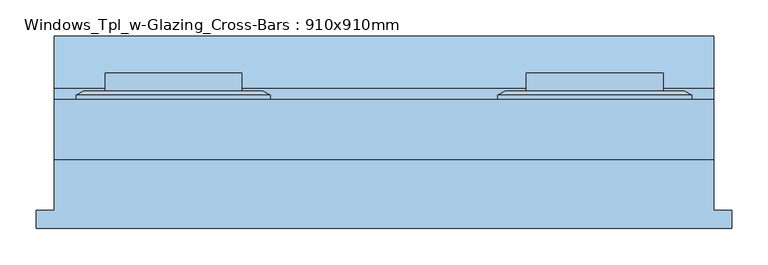
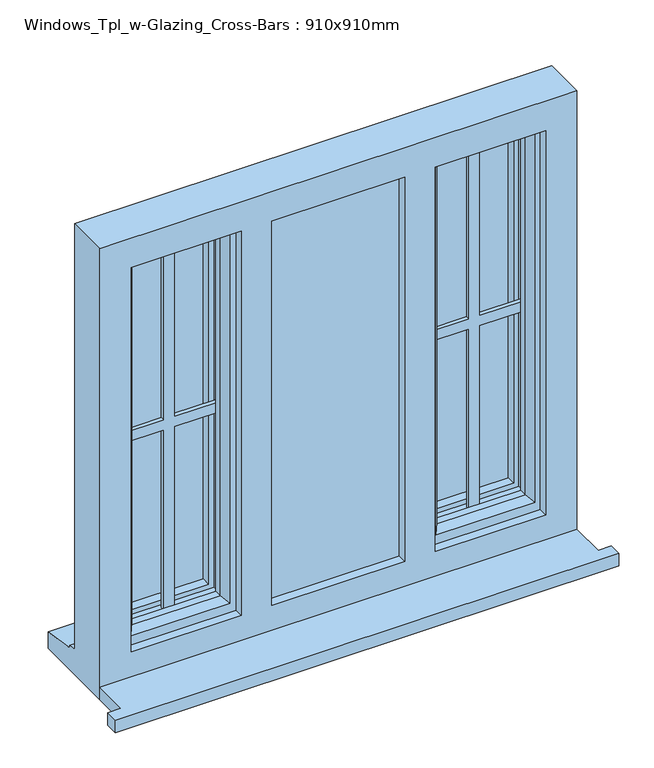
"""IFC4 building model written with IfcOpenShell, lengths in millimetres: window geometry, Windows_Tpl_w-Glazing_Cross-Bars : 910x910mm."""

from ifc_helpers import new_model, si_unit, frame, origin, place, context, project, spatial, polyline, outline, extrude, faceted_brep, source, transform, mapped, element, save


def windows_tpl_w_glazing_cross_bars_910x910mm_4aa0f884(model_context):
    return source(origin(), model_context, "Body", "SolidModel", [
        extrude(outline(polyline([(-906.6666667, -118.1434322), (-906.6666667, -93.1434322), (-881.6666667, -93.1434322), (-881.6666667, -22.9434322), (28.3333333, -22.9434322), (28.3333333, -93.1434322), (53.3333333, -93.1434322), (53.3333333, -118.1434322), (-906.6666667, -118.1434322)])), frame((0.0, 0.0, 1200.0), z_axis=(0.0, 0.0, 1.0), x_axis=(1.0, 0.0, 0.0)), (0.0, 0.0, 1.0), 25.0),
        faceted_brep([(-270.0, 60.0565678, 2080.0), (-270.0, 65.8300705, 2080.0), (-270.0, 65.8300705, 1253.0), (-270.0, 60.0565678, 1253.0), (-260.0, -4.9434322, 2070.0), (-260.0, 60.0565678, 2070.0), (-260.0, 60.0565678, 1263.0), (-260.0, -4.9434322, 1263.0), (-220.0, 9.5494677, 2030.0), (-230.1480377, -4.9434322, 2040.1480377), (-230.1480377, -4.9434322, 1292.8519623), (-220.0, 9.5494677, 1303.0), (-220.0, 24.0565678, 2030.0), (-220.0, 24.0565678, 1303.0), (-230.0, 48.0565678, 2040.0), (-230.0, 24.0565678, 2040.0), (-230.0, 24.0565678, 1293.0), (-230.0, 48.0565678, 1293.0), (-220.0, 65.8300705, 2030.0), (-220.0, 48.0565678, 2030.0), (-220.0, 48.0565678, 1303.0), (-220.0, 65.8300705, 1303.0), (-237.4457548, 71.6035732, 2047.4457548), (-237.4457548, 71.6035732, 1285.5542452), (-259.2153903, 71.6035732, 2069.2153903), (-259.2153903, 71.6035732, 1263.7846097), (-1.6666667, 65.8300705, 1253.0), (-1.6666667, 60.0565678, 1253.0), (-11.6666667, 60.0565678, 1263.0), (-11.6666667, -4.9434322, 1263.0), (-41.5186289, -4.9434322, 1292.8519623), (-51.6666667, 9.5494677, 1303.0), (-51.6666667, 24.0565678, 1303.0), (-41.6666667, 24.0565678, 1293.0), (-41.6666667, 48.0565678, 1293.0), (-51.6666667, 48.0565678, 1303.0), (-51.6666667, 65.8300705, 1303.0), (-34.2209119, 71.6035732, 1285.5542452), (-12.4512764, 71.6035732, 1263.7846097), (-1.6666667, 65.8300705, 2080.0), (-1.6666667, 60.0565678, 2080.0), (-11.6666667, 60.0565678, 2070.0), (-11.6666667, -4.9434322, 2070.0), (-41.5186289, -4.9434322, 2040.1480377), (-51.6666667, 9.5494677, 2030.0), (-51.6666667, 24.0565678, 2030.0), (-41.6666667, 24.0565678, 2040.0), (-41.6666667, 48.0565678, 2040.0), (-51.6666667, 48.0565678, 2030.0), (-51.6666667, 65.8300705, 2030.0), (-34.2209119, 71.6035732, 2047.4457548), (-12.4512764, 71.6035732, 2069.2153903)], [[[0, 1, 2, 3]], [[4, 5, 6, 7]], [[8, 9, 10, 11]], [[12, 8, 11, 13]], [[14, 15, 16, 17]], [[18, 19, 20, 21]], [[22, 18, 21, 23]], [[1, 24, 25, 2]], [[3, 2, 26, 27]], [[7, 6, 28, 29]], [[11, 10, 30, 31]], [[13, 11, 31, 32]], [[17, 16, 33, 34]], [[21, 20, 35, 36]], [[23, 21, 36, 37]], [[2, 25, 38, 26]], [[27, 26, 39, 40]], [[29, 28, 41, 42]], [[31, 30, 43, 44]], [[32, 31, 44, 45]], [[34, 33, 46, 47]], [[36, 35, 48, 49]], [[37, 36, 49, 50]], [[26, 38, 51, 39]], [[40, 39, 1, 0]], [[3, 27, 40, 0], [5, 41, 28, 6]], [[42, 41, 5, 4]], [[7, 29, 42, 4], [9, 43, 30, 10]], [[44, 43, 9, 8]], [[45, 44, 8, 12]], [[15, 46, 33, 16], [13, 32, 45, 12]], [[47, 46, 15, 14]], [[17, 34, 47, 14], [19, 48, 35, 20]], [[49, 48, 19, 18]], [[50, 49, 18, 22]], [[24, 51, 38, 25], [23, 37, 50, 22]], [[39, 51, 24, 1]]]),
        faceted_brep([(-583.3333333, 60.0565678, 2080.0), (-583.3333333, 65.8300705, 2080.0), (-851.6666667, 65.8300705, 2080.0), (-851.6666667, 60.0565678, 2080.0), (-593.3333333, -4.9434322, 2070.0), (-593.3333333, 60.0565678, 2070.0), (-841.6666667, 60.0565678, 2070.0), (-841.6666667, -4.9434322, 2070.0), (-633.3333333, 9.5494677, 2030.0), (-623.1852956, -4.9434322, 2040.1480377), (-811.8147044, -4.9434322, 2040.1480377), (-801.6666667, 9.5494677, 2030.0), (-633.3333333, 24.0565678, 2030.0), (-801.6666667, 24.0565678, 2030.0), (-623.3333333, 48.0565678, 2040.0), (-623.3333333, 24.0565678, 2040.0), (-811.6666667, 24.0565678, 2040.0), (-811.6666667, 48.0565678, 2040.0), (-633.3333333, 65.8300705, 2030.0), (-633.3333333, 48.0565678, 2030.0), (-801.6666667, 48.0565678, 2030.0), (-801.6666667, 65.8300705, 2030.0), (-615.8875785, 71.6035732, 2047.4457548), (-819.1124215, 71.6035732, 2047.4457548), (-594.117943, 71.6035732, 2069.2153903), (-840.882057, 71.6035732, 2069.2153903), (-851.6666667, 65.8300705, 1253.0), (-851.6666667, 60.0565678, 1253.0), (-841.6666667, 60.0565678, 1263.0), (-841.6666667, -4.9434322, 1263.0), (-811.8147044, -4.9434322, 1292.8519623), (-801.6666667, 9.5494677, 1303.0), (-801.6666667, 24.0565678, 1303.0), (-811.6666667, 24.0565678, 1293.0), (-811.6666667, 48.0565678, 1293.0), (-801.6666667, 48.0565678, 1303.0), (-801.6666667, 65.8300705, 1303.0), (-819.1124215, 71.6035732, 1285.5542452), (-840.882057, 71.6035732, 1263.7846097), (-583.3333333, 65.8300705, 1253.0), (-583.3333333, 60.0565678, 1253.0), (-593.3333333, 60.0565678, 1263.0), (-593.3333333, -4.9434322, 1263.0), (-623.1852956, -4.9434322, 1292.8519623), (-633.3333333, 9.5494677, 1303.0), (-633.3333333, 24.0565678, 1303.0), (-623.3333333, 24.0565678, 1293.0), (-623.3333333, 48.0565678, 1293.0), (-633.3333333, 48.0565678, 1303.0), (-633.3333333, 65.8300705, 1303.0), (-615.8875785, 71.6035732, 1285.5542452), (-594.117943, 71.6035732, 1263.7846097)], [[[0, 1, 2, 3]], [[4, 5, 6, 7]], [[8, 9, 10, 11]], [[12, 8, 11, 13]], [[14, 15, 16, 17]], [[18, 19, 20, 21]], [[22, 18, 21, 23]], [[1, 24, 25, 2]], [[3, 2, 26, 27]], [[7, 6, 28, 29]], [[11, 10, 30, 31]], [[13, 11, 31, 32]], [[17, 16, 33, 34]], [[21, 20, 35, 36]], [[23, 21, 36, 37]], [[2, 25, 38, 26]], [[27, 26, 39, 40]], [[0, 3, 27, 40], [41, 28, 6, 5]], [[29, 28, 41, 42]], [[4, 7, 29, 42], [43, 30, 10, 9]], [[31, 30, 43, 44]], [[32, 31, 44, 45]], [[46, 33, 16, 15], [12, 13, 32, 45]], [[34, 33, 46, 47]], [[14, 17, 34, 47], [48, 35, 20, 19]], [[36, 35, 48, 49]], [[37, 36, 49, 50]], [[51, 38, 25, 24], [22, 23, 37, 50]], [[26, 38, 51, 39]], [[40, 39, 1, 0]], [[42, 41, 5, 4]], [[44, 43, 9, 8]], [[45, 44, 8, 12]], [[47, 46, 15, 14]], [[49, 48, 19, 18]], [[50, 49, 18, 22]], [[39, 51, 24, 1]]]),
        extrude(outline(polyline([(1293.0, -145.8333333), (1293.0, -125.8333333), (1656.5, -125.8333333), (1656.5, -41.6666667), (1676.5, -41.6666667), (1676.5, -125.8333333), (2040.1480377, -125.8333333), (2040.1480377, -145.8333333), (1676.5, -145.8333333), (1676.5, -230.1480377), (1656.5, -230.1480377), (1656.5, -145.8333333), (1293.0, -145.8333333)])), frame((0.0, 32.0565678, 0.0), z_axis=(0.0, 1.0, 0.0), x_axis=(0.0, 0.0, 1.0)), (0.0, 0.0, 1.0), 8.0),
        extrude(outline(polyline([(1293.0, -727.5), (1293.0, -707.5), (1656.5, -707.5), (1656.5, -623.3333333), (1676.5, -623.3333333), (1676.5, -707.5), (2040.1480377, -707.5), (2040.1480377, -727.5), (1676.5, -727.5), (1676.5, -811.6666667), (1656.5, -811.6666667), (1656.5, -727.5), (1293.0, -727.5)])), frame((0.0, 32.0565678, 0.0), z_axis=(0.0, 1.0, 0.0), x_axis=(0.0, 0.0, 1.0)), (0.0, 0.0, 1.0), 8.0),
        extrude(outline(polyline([(1263.0, -436.6666667), (1263.0, -416.6666667), (1656.5, -416.6666667), (1656.5, -290.0), (1676.5, -290.0), (1676.5, -416.6666667), (2070.0, -416.6666667), (2070.0, -436.6666667), (1676.5, -436.6666667), (1676.5, -563.3333333), (1656.5, -563.3333333), (1656.5, -436.6666667), (1263.0, -436.6666667)])), frame((0.0, 3.0565678, 0.0), z_axis=(0.0, 1.0, 0.0), x_axis=(0.0, 0.0, 1.0)), (0.0, 0.0, 1.0), 8.0),
        faceted_brep([(28.3333333, -22.9434322, 2110.0), (-881.6666667, -22.9434322, 2110.0), (-881.6666667, -22.9434322, 1200.0), (28.3333333, -22.9434322, 1200.0), (-31.6666667, -22.9434322, 2050.0), (-31.6666667, -22.9434322, 1275.0), (-242.0, -22.9434322, 1275.0), (-242.0, -22.9434322, 2050.0), (-300.0, -22.9434322, 2050.0), (-300.0, -22.9434322, 1275.0), (-553.3333333, -22.9434322, 1275.0), (-553.3333333, -22.9434322, 2050.0), (-611.3333333, -22.9434322, 2050.0), (-611.3333333, -22.9434322, 1275.0), (-821.6666667, -22.9434322, 1275.0), (-821.6666667, -22.9434322, 2050.0), (-881.6666667, 60.0565678, 2110.0), (-881.6666667, 60.0565678, 1251.0), (-881.6666667, 75.0565678, 1249.68767), (-881.6666667, 75.0565678, 1244.7449676), (-881.6666667, 147.5565678, 1233.8088847), (-881.6666667, 147.5565678, 1200.0), (28.3333333, 60.0565678, 2110.0), (28.3333333, 60.0565678, 1251.0), (-841.6666667, 60.0565678, 2070.0), (-841.6666667, 60.0565678, 1263.0), (-593.3333333, 60.0565678, 1263.0), (-593.3333333, 60.0565678, 2070.0), (-553.3333333, 60.0565678, 2070.0), (-553.3333333, 60.0565678, 1263.0), (-300.0, 60.0565678, 1263.0), (-300.0, 60.0565678, 2070.0), (-260.0, 60.0565678, 2070.0), (-260.0, 60.0565678, 1263.0), (-11.6666667, 60.0565678, 1263.0), (-11.6666667, 60.0565678, 2070.0), (-841.6666667, -4.9434322, 2070.0), (-841.6666667, -4.9434322, 1263.0), (-563.3333333, -4.9434322, 2070.0), (-290.0, -4.9434322, 2070.0), (-290.0, -4.9434322, 1263.0), (-563.3333333, -4.9434322, 1263.0), (-300.0, -4.9434322, 2050.0), (-553.3333333, -4.9434322, 2050.0), (-553.3333333, -4.9434322, 1275.0), (-300.0, -4.9434322, 1275.0), (-260.0, -4.9434322, 2070.0), (-11.6666667, -4.9434322, 2070.0), (-11.6666667, -4.9434322, 1263.0), (-260.0, -4.9434322, 1263.0), (-31.6666667, -4.9434322, 2050.0), (-242.0, -4.9434322, 2050.0), (-242.0, -4.9434322, 1275.0), (-31.6666667, -4.9434322, 1275.0), (-593.3333333, -4.9434322, 2070.0), (-593.3333333, -4.9434322, 1263.0), (-611.3333333, -4.9434322, 2050.0), (-821.6666667, -4.9434322, 2050.0), (-821.6666667, -4.9434322, 1275.0), (-611.3333333, -4.9434322, 1275.0), (-553.3333333, 19.0565678, 2070.0), (-300.0, 19.0565678, 2070.0), (-290.0, 19.0565678, 2070.0), (-563.3333333, 19.0565678, 2070.0), (28.3333333, 147.5565678, 1200.0), (28.3333333, 147.5565678, 1233.8088847), (28.3333333, 75.0565678, 1244.7449676), (28.3333333, 75.0565678, 1249.68767), (-553.3333333, 19.0565678, 1263.0), (-563.3333333, 19.0565678, 1263.0), (-290.0, 19.0565678, 1263.0), (-300.0, 19.0565678, 1263.0)], [[[0, 1, 2, 3], [4, 5, 6, 7], [8, 9, 10, 11], [12, 13, 14, 15]], [[2, 1, 16, 17, 18, 19, 20, 21]], [[17, 16, 22, 23], [24, 25, 26, 27], [28, 29, 30, 31], [32, 33, 34, 35]], [[25, 24, 36, 37]], [[38, 39, 40, 41], [42, 43, 44, 45]], [[46, 47, 48, 49], [50, 51, 52, 53]], [[36, 54, 55, 37], [56, 57, 58, 59]], [[57, 15, 14, 58]], [[1, 0, 22, 16]], [[36, 24, 27, 54]], [[35, 47, 46, 32]], [[60, 28, 31, 61, 62, 39, 38, 63]], [[15, 57, 56, 12]], [[50, 4, 7, 51]], [[11, 43, 42, 8]], [[23, 22, 0, 3, 64, 65, 66, 67]], [[35, 34, 48, 47]], [[4, 50, 53, 5]], [[43, 11, 10, 44]], [[12, 56, 59, 13]], [[27, 26, 55, 54]], [[29, 28, 60, 68]], [[68, 60, 63, 69]], [[69, 63, 38, 41]], [[62, 70, 40, 39]], [[70, 62, 61, 71]], [[71, 61, 31, 30]], [[33, 32, 46, 49]], [[51, 7, 6, 52]], [[8, 42, 45, 9]], [[64, 3, 2, 21]], [[65, 64, 21, 20]], [[66, 65, 20, 19]], [[67, 66, 19, 18]], [[23, 67, 18, 17]], [[26, 25, 37, 55]], [[34, 33, 49, 48]], [[41, 40, 70, 71, 30, 29, 68, 69]], [[6, 5, 53, 52]], [[45, 44, 10, 9]], [[59, 58, 14, 13]]]),
        extrude(outline(polyline([(-563.3333333, 19.0565678), (-290.0, 19.0565678), (-290.0, -4.9434322), (-563.3333333, -4.9434322), (-563.3333333, 19.0565678)])), frame((0.0, 0.0, 1263.0), z_axis=(0.0, 0.0, 1.0), x_axis=(1.0, 0.0, 0.0)), (0.0, 0.0, 1.0), 807.0),
        extrude(outline(polyline([(-623.3333333, 72.4565678), (-811.6666667, 72.4565678), (-811.6666667, 96.4565678), (-623.3333333, 96.4565678), (-623.3333333, 72.4565678)])), frame((0.0, 0.0, 1293.0), z_axis=(0.0, 0.0, 1.0), x_axis=(1.0, 0.0, 0.0)), (0.0, 0.0, 1.0), 747.0),
        extrude(outline(polyline([(-41.5186289, 72.4565678), (-230.1480377, 72.4565678), (-230.1480377, 96.4565678), (-41.5186289, 96.4565678), (-41.5186289, 72.4565678)])), frame((0.0, 0.0, 1292.8519623), z_axis=(0.0, 0.0, 1.0), x_axis=(1.0, 0.0, 0.0)), (0.0, 0.0, 1.0), 747.2960754),
    ])


if __name__ == "__main__":
    model = new_model("IFC4")
    model_context = context("Model", 3, world=origin())
    ifc_project = project(units=[si_unit("LENGTHUNIT", "METRE", prefix="MILLI")], contexts=[model_context])
    site = spatial("IfcSite", under=ifc_project)
    building = spatial("IfcBuilding", under=site)
    placement = place(None, origin())
    windows_tpl_w_glazing_cross_bars_910x910mm_shape = windows_tpl_w_glazing_cross_bars_910x910mm_4aa0f884(model_context)
    element("IfcWindow", 1, ObjectType="Windows_Tpl_w-Glazing_Cross-Bars : 910x910mm", at=placement, inside=building, context=model_context, shape_type="MappedRepresentation", body=[
        mapped(windows_tpl_w_glazing_cross_bars_910x910mm_shape, transform((0.0, 0.0, 0.0), x_axis=(1.0, 0.0, 0.0), y_axis=(0.0, 1.0, 0.0), z_axis=(0.0, 0.0, 1.0))),
    ])
    save(model, "model.ifc")

# Revit data of these elements
# Type "Windows_Tpl_w-Glazing_Cross-Bars : 910x910mm"
#   Type Mark = "24"
#   Operation = "TriplePanelVertical"
#   Construction Type Id = "GSP4R"
#   Manufacturer = "Revit"
#   Keynote = "L10"
#   Analytic Construction = "1/8 in Pilkington single glazing"
#   Wrap Layers (Ext) from Ext = 0' - 4.03543"
#   Wrap Layers (Int) from Ext = 0' - 6.98819"
#   Window Board Projection = 0' - 0.98425"
#   Window Board Extension = 0' - 0.98425"
#   Visual Light Transmittance = 0.9
#   Solar Heat Gain Coefficient = 0.78
#   Rough Width = 2' - 11.82677"
#   Rough Height = 2' - 11.82677"
#   Height = 2' - 11.82677"
#   Width = 2' - 11.82677"
#   Heat Transfer Coefficient (U) = 0.6496 BTU/(h·ft²·°F)
#   Glazing Thickness = 0' - 0.94488"
#   Glazing Bar Thickness = 0' - 0.7874"
#   FrameOffset - External = 0' - 1.9685"
#   Frame Depth = 0' - 2.55906"
#   Default Head Height = 6' - 11.07087"
#   Cill Depth = 0' - 3.44488"
#   Cavity Closer Width = 0' - 1.9685"
#   Cavity Closer Offset from Ext = 0' - 4.03543"
#   Cavity Closer Depth = 0' - 3.34646"
#   Vis - Glazing Bars = yes
#   Vis - Cavity Closers = yes
#   Define Thermal Properties by = 1
#   Material Trim = Window Frame
#   Material Glazing Bars = Window Frame
#   Material Glass = Glass
#   Material Frame = Window Frame
#   Wall Closure = (empty or 0)
# Element 1 (IfcWindow, "Windows_Tpl_w-Glazing_Cross-Bars : 910x910mm")
#   Materials on its faces: "Window Frame", "Glass"
# Materials
#   "Window Frame": colour RGB 249 249 249, transparency 0
#   "Glass": class "Glass", colour RGB 0 128 192, transparency 0.75, Description = "Soda Lime Glass", Cost = 0
